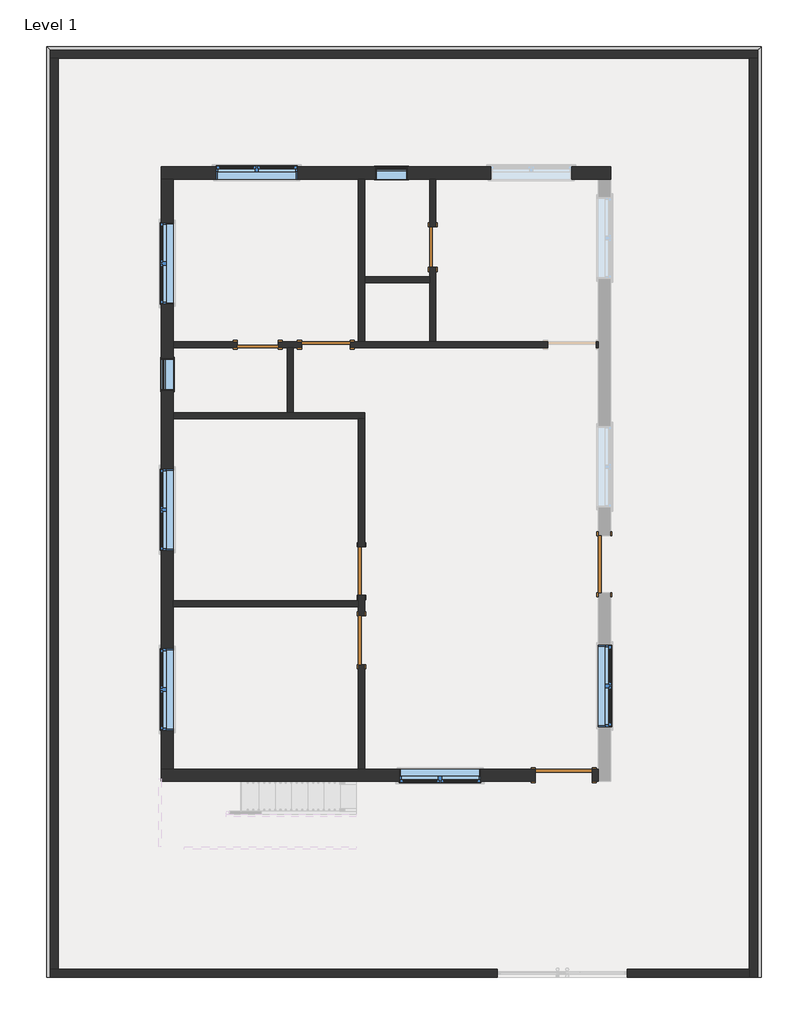
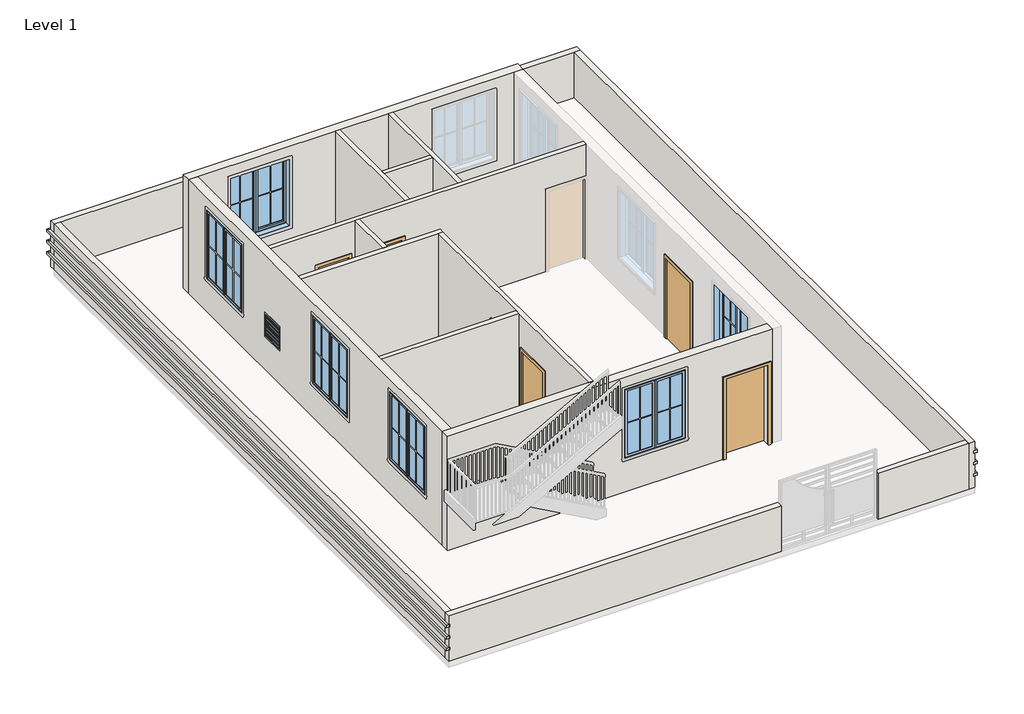
# One storey, part 1 of 3: 16 walls, 8 windows, 7 doors, 3 proxies.
"""IFC4 building model written with IfcOpenShell, lengths in millimetres."""

from ifc_helpers import new_model, si_unit, frame, origin, origin_with_axes, place, context, project, spatial, polyline, outline, extrude, faceted_brep, transform, mapped, element, save
from components import door_78caadf7, single_flush_door_3_e5f9f3c4, single_flush_door_3_305aa2a5, door_9d399b00, door_0848dd25, window_casement_double_win_5_f93960c7, window_f2d8fef0

model = new_model("IFC4")

# Units and contexts
model_context = context("Model", 3, world=origin())
ifc_project = project(units=[si_unit("LENGTHUNIT", "METRE", prefix="MILLI")], contexts=[model_context])

# Site, building, storey
site = spatial("IfcSite", under=ifc_project)
building = spatial("IfcBuilding", under=site)
storey = spatial("IfcBuildingStorey", under=building, Name="Level 1", Elevation=0.0)

# Proxies
placement = place(None, origin())
element("IfcBuildingElementProxy", 1, Name="Reveal", ObjectType="Reveal", at=placement, inside=storey, context=model_context, shape_type="SweptSolid", body=[
    extrude(outline(polyline([(-7520.8438076, -8973.0750537), (-7612.9188076, -8973.0750537), (-7612.9188076, 8467.1999463), (-7520.8438076, 8375.1249463), (-7520.8438076, -8973.0750537)])), frame((0.0, 0.0, 304.8), z_axis=(0.0, 0.0, 1.0), x_axis=(1.0, 0.0, 0.0)), (0.0, 0.0, 1.0), 67.7333333),
    extrude(outline(polyline([(-7520.8438076, 8375.1249463), (-7612.9188076, 8467.1999463), (5779.2311924, 8467.1999463), (5687.1561924, 8375.1249463), (-7520.8438076, 8375.1249463)])), frame((0.0, 0.0, 304.8), z_axis=(0.0, 0.0, 1.0), x_axis=(1.0, 0.0, 0.0)), (0.0, 0.0, 1.0), 67.7333333),
    extrude(outline(polyline([(5687.1561924, 8375.1249463), (5779.2311924, 8467.1999463), (5779.2311924, -8973.0750537), (5687.1561924, -8973.0750537), (5687.1561924, 8375.1249463)])), frame((0.0, 0.0, 304.8), z_axis=(0.0, 0.0, 1.0), x_axis=(1.0, 0.0, 0.0)), (0.0, 0.0, 1.0), 67.7333333),
])
element("IfcBuildingElementProxy", 2, Name="Reveal", ObjectType="Reveal", at=placement, inside=storey, context=model_context, shape_type="SweptSolid", body=[
    extrude(outline(polyline([(-7520.8438076, -8973.0750537), (-7612.9188076, -8973.0750537), (-7612.9188076, 8467.1999463), (-7520.8438076, 8375.1249463), (-7520.8438076, -8973.0750537)])), frame((0.0, 0.0, 609.6), z_axis=(0.0, 0.0, 1.0), x_axis=(1.0, 0.0, 0.0)), (0.0, 0.0, 1.0), 67.7333333),
    extrude(outline(polyline([(-7520.8438076, 8375.1249463), (-7612.9188076, 8467.1999463), (5779.2311924, 8467.1999463), (5687.1561924, 8375.1249463), (-7520.8438076, 8375.1249463)])), frame((0.0, 0.0, 609.6), z_axis=(0.0, 0.0, 1.0), x_axis=(1.0, 0.0, 0.0)), (0.0, 0.0, 1.0), 67.7333333),
    extrude(outline(polyline([(5687.1561924, 8375.1249463), (5779.2311924, 8467.1999463), (5779.2311924, -8973.0750537), (5687.1561924, -8973.0750537), (5687.1561924, 8375.1249463)])), frame((0.0, 0.0, 609.6), z_axis=(0.0, 0.0, 1.0), x_axis=(1.0, 0.0, 0.0)), (0.0, 0.0, 1.0), 67.7333333),
])
element("IfcBuildingElementProxy", 3, Name="Reveal", ObjectType="Reveal", at=placement, inside=storey, context=model_context, shape_type="SweptSolid", body=[
    extrude(outline(polyline([(-7520.8438076, -8973.0750537), (-7612.9188076, -8973.0750537), (-7612.9188076, 8467.1999463), (-7520.8438076, 8375.1249463), (-7520.8438076, -8973.0750537)])), frame((0.0, 0.0, 914.4), z_axis=(0.0, 0.0, 1.0), x_axis=(1.0, 0.0, 0.0)), (0.0, 0.0, 1.0), 67.7333333),
    extrude(outline(polyline([(-7520.8438076, 8375.1249463), (-7612.9188076, 8467.1999463), (5779.2311924, 8467.1999463), (5687.1561924, 8375.1249463), (-7520.8438076, 8375.1249463)])), frame((0.0, 0.0, 914.4), z_axis=(0.0, 0.0, 1.0), x_axis=(1.0, 0.0, 0.0)), (0.0, 0.0, 1.0), 67.7333333),
    extrude(outline(polyline([(5687.1561924, 8375.1249463), (5779.2311924, 8467.1999463), (5779.2311924, -8973.0750537), (5687.1561924, -8973.0750537), (5687.1561924, 8375.1249463)])), frame((0.0, 0.0, 914.4), z_axis=(0.0, 0.0, 1.0), x_axis=(1.0, 0.0, 0.0)), (0.0, 0.0, 1.0), 67.7333333),
])

# Doors
door_shape = door_78caadf7(model_context)
element("IfcDoor", 4, ObjectType="Single-Flush : DOOR 2'6\"", at=placement, inside=storey, context=model_context, shape_type="MappedRepresentation", body=[
    mapped(door_shape, transform((-377.1698569, 4707.5566963, 0.0), x_axis=(0.0, -1.0, 0.0), y_axis=(1.0, 0.0, 0.0), z_axis=(0.0, 0.0, 1.0))),
])
element("IfcDoor", 5, ObjectType="Single-Flush : DOOR 2'6\"", at=placement, inside=storey, context=model_context, shape_type="MappedRepresentation", body=[
    mapped(door_shape, transform((-3653.7698569, 2878.7566963, 0.0), x_axis=(1.0, 0.0, 0.0), y_axis=(0.0, 1.0, 0.0), z_axis=(0.0, 0.0, 1.0))),
])
single_flush_door_3_shape = single_flush_door_3_e5f9f3c4(model_context)
element("IfcDoor", 6, ObjectType="Single-Flush : DOOR 3'", at=placement, inside=storey, context=model_context, shape_type="MappedRepresentation", body=[
    mapped(single_flush_door_3_shape, transform((-2377.4198569, 2878.7566963, 0.0), x_axis=(1.0, 0.0, 0.0), y_axis=(0.0, 1.0, 0.0), z_axis=(0.0, 0.0, 1.0))),
])
element("IfcDoor", 7, ObjectType="Single-Flush : DOOR 3'", at=placement, inside=storey, context=model_context, shape_type="MappedRepresentation", body=[
    mapped(single_flush_door_3_shape, transform((-1710.6698569, -2658.4433037, 0.0), x_axis=(0.0, 1.0, 0.0), y_axis=(-1.0, 0.0, 0.0), z_axis=(0.0, 0.0, 1.0))),
])
single_flush_door_3_2_shape = single_flush_door_3_305aa2a5(model_context)
element("IfcDoor", 8, ObjectType="Single-Flush : DOOR 3'", at=placement, inside=storey, context=model_context, shape_type="MappedRepresentation", body=[
    mapped(single_flush_door_3_2_shape, transform((-1710.6698569, -1363.0433037, 0.0), x_axis=(0.0, -1.0, 0.0), y_axis=(1.0, 0.0, 0.0), z_axis=(0.0, 0.0, 1.0))),
])
door_2_shape = door_9d399b00(model_context)
element("IfcDoor", 9, ObjectType="Single-Flush : DOOR 3'6\"", at=placement, inside=storey, context=model_context, shape_type="MappedRepresentation", body=[
    mapped(door_2_shape, transform((2080.2801431, -5192.0933037, 0.0), x_axis=(1.0, 0.0, 0.0), y_axis=(0.0, 1.0, 0.0), z_axis=(0.0, 0.0, 1.0))),
])
door_3_shape = door_0848dd25(model_context)
element("IfcDoor", 10, ObjectType="Single-Flush : DOOR 3'6\"", at=placement, inside=storey, context=model_context, shape_type="MappedRepresentation", body=[
    mapped(door_3_shape, transform((2842.2801431, -1236.0433037, 0.0), x_axis=(0.0, -1.0, 0.0), y_axis=(1.0, 0.0, 0.0), z_axis=(0.0, 0.0, 1.0))),
])

# Walls
element("IfcWall", 11, ObjectType="CMD 6\"", at=placement, inside=storey, context=model_context, shape_type="Brep", body=[
    faceted_brep([(-7546.2438076, 8248.1249463, 0.0), (-7393.8438076, 8248.1249463, 0.0), (5560.1561924, 8248.1249463, 0.0), (5712.5561924, 8248.1249463, 0.0), (5712.5561924, 8248.1249463, 304.8), (5687.1561924, 8248.1249463, 304.8), (5687.1561924, 8248.1249463, 372.5333333), (5712.5561924, 8248.1249463, 372.5333333), (5712.5561924, 8248.1249463, 609.6), (5687.1561924, 8248.1249463, 609.6), (5687.1561924, 8248.1249463, 677.3333333), (5712.5561924, 8248.1249463, 677.3333333), (5712.5561924, 8248.1249463, 914.4), (5687.1561924, 8248.1249463, 914.4), (5687.1561924, 8248.1249463, 982.1333333), (5712.5561924, 8248.1249463, 982.1333333), (5712.5561924, 8248.1249463, 1219.2), (5560.1561924, 8248.1249463, 1219.2), (-7393.8438076, 8248.1249463, 1219.2), (-7546.2438076, 8248.1249463, 1219.2), (-7546.2438076, 8248.1249463, 982.1333333), (-7520.8438076, 8248.1249463, 982.1333333), (-7520.8438076, 8248.1249463, 914.4), (-7546.2438076, 8248.1249463, 914.4), (-7546.2438076, 8248.1249463, 677.3333333), (-7520.8438076, 8248.1249463, 677.3333333), (-7520.8438076, 8248.1249463, 609.6), (-7546.2438076, 8248.1249463, 609.6), (-7546.2438076, 8248.1249463, 372.5333333), (-7520.8438076, 8248.1249463, 372.5333333), (-7520.8438076, 8248.1249463, 304.8), (-7546.2438076, 8248.1249463, 304.8), (5712.5561924, 8400.5249463, 0.0), (-7546.2438076, 8400.5249463, 0.0), (-7546.2438076, 8400.5249463, 304.8), (5712.5561924, 8400.5249463, 304.8), (-7546.2438076, 8400.5249463, 1219.2), (5712.5561924, 8400.5249463, 1219.2), (5712.5561924, 8400.5249463, 982.1333333), (-7546.2438076, 8400.5249463, 982.1333333), (5712.5561924, 8400.5249463, 372.5333333), (-7546.2438076, 8400.5249463, 372.5333333), (-7546.2438076, 8400.5249463, 609.6), (5712.5561924, 8400.5249463, 609.6), (5712.5561924, 8400.5249463, 677.3333333), (-7546.2438076, 8400.5249463, 677.3333333), (-7546.2438076, 8400.5249463, 914.4), (5712.5561924, 8400.5249463, 914.4), (5687.1561924, 8375.1249463, 372.5333333), (-7520.8438076, 8375.1249463, 372.5333333), (-7520.8438076, 8375.1249463, 304.8), (5687.1561924, 8375.1249463, 304.8), (5687.1561924, 8375.1249463, 677.3333333), (-7520.8438076, 8375.1249463, 677.3333333), (-7520.8438076, 8375.1249463, 609.6), (5687.1561924, 8375.1249463, 609.6), (5687.1561924, 8375.1249463, 982.1333333), (-7520.8438076, 8375.1249463, 982.1333333), (-7520.8438076, 8375.1249463, 914.4), (5687.1561924, 8375.1249463, 914.4)], [[[0, 1, 2, 3, 4, 5, 6, 7, 8, 9, 10, 11, 12, 13, 14, 15, 16, 17, 18, 19, 20, 21, 22, 23, 24, 25, 26, 27, 28, 29, 30, 31]], [[32, 33, 34, 35]], [[36, 37, 38, 39]], [[40, 41, 42, 43]], [[44, 45, 46, 47]], [[3, 2, 1, 0, 33, 32]], [[19, 18, 17, 16, 37, 36]], [[3, 32, 35, 4]], [[37, 16, 15, 38]], [[7, 40, 43, 8]], [[11, 44, 47, 12]], [[19, 36, 39, 20]], [[33, 0, 31, 34]], [[41, 28, 27, 42]], [[45, 24, 23, 46]], [[48, 49, 29, 28, 41, 40, 7, 6]], [[50, 51, 5, 4, 35, 34, 31, 30]], [[49, 50, 30, 29]], [[49, 48, 51, 50]], [[51, 48, 6, 5]], [[52, 53, 25, 24, 45, 44, 11, 10]], [[54, 55, 9, 8, 43, 42, 27, 26]], [[53, 54, 26, 25]], [[53, 52, 55, 54]], [[55, 52, 10, 9]], [[56, 57, 21, 20, 39, 38, 15, 14]], [[58, 59, 13, 12, 47, 46, 23, 22]], [[57, 58, 22, 21]], [[57, 56, 59, 58]], [[59, 56, 14, 13]]]),
])
element("IfcWall", 12, ObjectType="CMD 6\"", at=placement, inside=storey, context=model_context, shape_type="Brep", body=[
    faceted_brep([(5560.1561924, 8248.1249463, 0.0), (5560.1561924, -8820.6750537, 0.0), (5560.1561924, -8973.0750537, 0.0), (5560.1561924, -8973.0750537, 1219.2), (5560.1561924, -8820.6750537, 1219.2), (5560.1561924, 8248.1249463, 1219.2), (5712.5561924, -8973.0750537, 0.0), (5712.5561924, 8248.1249463, 0.0), (5712.5561924, 8248.1249463, 304.8), (5712.5561924, -8973.0750537, 304.8), (5712.5561924, 8248.1249463, 1219.2), (5712.5561924, -8973.0750537, 1219.2), (5712.5561924, -8973.0750537, 982.1333333), (5712.5561924, 8248.1249463, 982.1333333), (5712.5561924, -8973.0750537, 372.5333333), (5712.5561924, 8248.1249463, 372.5333333), (5712.5561924, 8248.1249463, 609.6), (5712.5561924, -8973.0750537, 609.6), (5712.5561924, -8973.0750537, 677.3333333), (5712.5561924, 8248.1249463, 677.3333333), (5712.5561924, 8248.1249463, 914.4), (5712.5561924, -8973.0750537, 914.4), (5687.1561924, 8248.1249463, 982.1333333), (5687.1561924, 8248.1249463, 914.4), (5687.1561924, 8248.1249463, 677.3333333), (5687.1561924, 8248.1249463, 609.6), (5687.1561924, 8248.1249463, 372.5333333), (5687.1561924, 8248.1249463, 304.8), (5687.1561924, -8973.0750537, 304.8), (5687.1561924, -8973.0750537, 372.5333333), (5687.1561924, -8973.0750537, 609.6), (5687.1561924, -8973.0750537, 677.3333333), (5687.1561924, -8973.0750537, 914.4), (5687.1561924, -8973.0750537, 982.1333333)], [[[0, 1, 2, 3, 4, 5]], [[6, 7, 8, 9]], [[10, 11, 12, 13]], [[14, 15, 16, 17]], [[18, 19, 20, 21]], [[2, 1, 0, 7, 6]], [[5, 4, 3, 11, 10]], [[0, 5, 10, 13, 22, 23, 20, 19, 24, 25, 16, 15, 26, 27, 8, 7]], [[3, 2, 6, 9, 28, 29, 14, 17, 30, 31, 18, 21, 32, 33, 12, 11]], [[29, 26, 15, 14]], [[27, 28, 9, 8]], [[26, 29, 28, 27]], [[31, 24, 19, 18]], [[25, 30, 17, 16]], [[24, 31, 30, 25]], [[33, 22, 13, 12]], [[23, 32, 21, 20]], [[22, 33, 32, 23]]]),
])
element("IfcWall", 13, ObjectType="CMD 6\"", at=placement, inside=storey, context=model_context, shape_type="SweptSolid", body=[
    extrude(outline(polyline([(3274.1561924, -8820.6750537), (5560.1561924, -8820.6750537), (5560.1561924, -8973.0750537), (3274.1561924, -8973.0750537), (3274.1561924, -8820.6750537)])), origin_with_axes(), (0.0, 0.0, 1.0), 1219.2),
])
element("IfcWall", 14, ObjectType="CMD 6\"", at=placement, inside=storey, context=model_context, shape_type="SweptSolid", body=[
    extrude(outline(polyline([(0.0, -7393.8438076), (1219.2, -7393.8438076), (1219.2, -7546.2438076), (982.1333333, -7546.2438076), (982.1333333, -7520.8438076), (914.4, -7520.8438076), (914.4, -7546.2438076), (677.3333333, -7546.2438076), (677.3333333, -7520.8438076), (609.6, -7520.8438076), (609.6, -7546.2438076), (372.5333333, -7546.2438076), (372.5333333, -7520.8438076), (304.8, -7520.8438076), (304.8, -7546.2438076), (0.0, -7546.2438076), (0.0, -7393.8438076)])), frame((0.0, -8820.6750537, 0.0), z_axis=(0.0, 1.0, 0.0), x_axis=(0.0, 0.0, 1.0)), (0.0, 0.0, 1.0), 17068.8),
])
element("IfcWall", 15, ObjectType="CMD 6\"", at=placement, inside=storey, context=model_context, shape_type="Brep", body=[
    faceted_brep([(835.7561924, -8820.6750537, 0.0), (-7393.8438076, -8820.6750537, 0.0), (-7546.2438076, -8820.6750537, 0.0), (-7546.2438076, -8820.6750537, 304.8), (-7520.8438076, -8820.6750537, 304.8), (-7520.8438076, -8820.6750537, 372.5333333), (-7546.2438076, -8820.6750537, 372.5333333), (-7546.2438076, -8820.6750537, 609.6), (-7520.8438076, -8820.6750537, 609.6), (-7520.8438076, -8820.6750537, 677.3333333), (-7546.2438076, -8820.6750537, 677.3333333), (-7546.2438076, -8820.6750537, 914.4), (-7520.8438076, -8820.6750537, 914.4), (-7520.8438076, -8820.6750537, 982.1333333), (-7546.2438076, -8820.6750537, 982.1333333), (-7546.2438076, -8820.6750537, 1219.2), (-7393.8438076, -8820.6750537, 1219.2), (835.7561924, -8820.6750537, 1219.2), (-7546.2438076, -8973.0750537, 0.0), (835.7561924, -8973.0750537, 0.0), (835.7561924, -8973.0750537, 1219.2), (-7546.2438076, -8973.0750537, 1219.2), (-7546.2438076, -8973.0750537, 982.1333333), (-7520.8438076, -8973.0750537, 982.1333333), (-7520.8438076, -8973.0750537, 914.4), (-7546.2438076, -8973.0750537, 914.4), (-7546.2438076, -8973.0750537, 677.3333333), (-7520.8438076, -8973.0750537, 677.3333333), (-7520.8438076, -8973.0750537, 609.6), (-7546.2438076, -8973.0750537, 609.6), (-7546.2438076, -8973.0750537, 372.5333333), (-7520.8438076, -8973.0750537, 372.5333333), (-7520.8438076, -8973.0750537, 304.8), (-7546.2438076, -8973.0750537, 304.8)], [[[0, 1, 2, 3, 4, 5, 6, 7, 8, 9, 10, 11, 12, 13, 14, 15, 16, 17]], [[18, 19, 20, 21, 22, 23, 24, 25, 26, 27, 28, 29, 30, 31, 32, 33]], [[2, 1, 0, 19, 18]], [[17, 16, 15, 21, 20]], [[0, 17, 20, 19]], [[2, 18, 33, 3]], [[21, 15, 14, 22]], [[6, 30, 29, 7]], [[10, 26, 25, 11]], [[5, 31, 30, 6]], [[32, 4, 3, 33]], [[31, 5, 4, 32]], [[9, 27, 26, 10]], [[28, 8, 7, 29]], [[27, 9, 8, 28]], [[13, 23, 22, 14]], [[24, 12, 11, 25]], [[23, 13, 12, 24]]]),
])
element("IfcWall", 16, ObjectType="WALL 4.5\"", at=placement, inside=storey, context=model_context, shape_type="Brep", body=[
    faceted_brep([(2689.8801431, 2821.6066963, 2133.6), (2689.8801431, 2821.6066963, 0.0), (2727.9801431, 2821.6066963, 0.0), (2727.9801431, 2821.6066963, 3048.0), (-2987.0198569, 2821.6066963, 3048.0), (-3101.3198569, 2821.6066963, 3048.0), (-5234.9198569, 2821.6066963, 3048.0), (-5234.9198569, 2821.6066963, 0.0), (-4034.7698569, 2821.6066963, 0.0), (-4034.7698569, 2821.6066963, 2133.6), (-3272.7698569, 2821.6066963, 2133.6), (-3272.7698569, 2821.6066963, 0.0), (-3101.3198569, 2821.6066963, 0.0), (-2987.0198569, 2821.6066963, 0.0), (-2834.6198569, 2821.6066963, 0.0), (-2834.6198569, 2821.6066963, 2133.6), (-1920.2198569, 2821.6066963, 2133.6), (-1920.2198569, 2821.6066963, 0.0), (1775.4801431, 2821.6066963, 0.0), (1775.4801431, 2821.6066963, 2133.6), (2727.9801431, 2935.9066963, 0.0), (2689.8801431, 2935.9066963, 0.0), (2689.8801431, 2935.9066963, 2133.6), (1775.4801431, 2935.9066963, 2133.6), (1775.4801431, 2935.9066963, 0.0), (-320.0198569, 2935.9066963, 0.0), (-434.3198569, 2935.9066963, 0.0), (-1653.5198569, 2935.9066963, 0.0), (-1767.8198569, 2935.9066963, 0.0), (-1920.2198569, 2935.9066963, 0.0), (-1920.2198569, 2935.9066963, 2133.6), (-2834.6198569, 2935.9066963, 2133.6), (-2834.6198569, 2935.9066963, 0.0), (-3272.7698569, 2935.9066963, 0.0), (-3272.7698569, 2935.9066963, 2133.6), (-4034.7698569, 2935.9066963, 2133.6), (-4034.7698569, 2935.9066963, 0.0), (-5234.9198569, 2935.9066963, 0.0), (-5234.9198569, 2935.9066963, 3048.0), (-1767.8198569, 2935.9066963, 3048.0), (-1653.5198569, 2935.9066963, 3048.0), (-434.3198569, 2935.9066963, 3048.0), (-320.0198569, 2935.9066963, 3048.0), (2727.9801431, 2935.9066963, 3048.0)], [[[0, 1, 2, 3, 4, 5, 6, 7, 8, 9, 10, 11, 12, 13, 14, 15, 16, 17, 18, 19]], [[20, 21, 22, 23, 24, 25, 26, 27, 28, 29, 30, 31, 32, 33, 34, 35, 36, 37, 38, 39, 40, 41, 42, 43]], [[8, 7, 37, 36]], [[14, 13, 12, 11, 33, 32]], [[18, 17, 29, 28, 27, 26, 25, 24]], [[2, 1, 21, 20]], [[3, 2, 20, 43]], [[7, 6, 38, 37]], [[34, 33, 11, 10]], [[35, 34, 10, 9]], [[36, 35, 9, 8]], [[30, 29, 17, 16]], [[31, 30, 16, 15]], [[32, 31, 15, 14]], [[22, 21, 1, 0]], [[23, 22, 0, 19]], [[24, 23, 19, 18]], [[6, 5, 4, 3, 43, 42, 41, 40, 39, 38]]]),
])
element("IfcWall", 17, ObjectType="WALL 4.5\"", at=placement, inside=storey, context=model_context, shape_type="Brep", body=[
    faceted_brep([(-1767.8198569, 5983.9066963, 0.0), (-1767.8198569, 2935.9066963, 0.0), (-1767.8198569, 2935.9066963, 3048.0), (-1767.8198569, 5983.9066963, 3048.0), (-1653.5198569, 5983.9066963, 0.0), (-1653.5198569, 5983.9066963, 3048.0), (-1653.5198569, 4155.1066963, 3048.0), (-1653.5198569, 4040.8066963, 3048.0), (-1653.5198569, 2935.9066963, 3048.0), (-1653.5198569, 2935.9066963, 0.0), (-1653.5198569, 4040.8066963, 0.0), (-1653.5198569, 4155.1066963, 0.0)], [[[0, 1, 2, 3]], [[4, 5, 6, 7, 8, 9, 10, 11]], [[1, 0, 4, 11, 10, 9]], [[0, 3, 5, 4]], [[2, 1, 9, 8]], [[3, 2, 8, 7, 6, 5]]]),
])
element("IfcWall", 18, ObjectType="WALL 4.5\"", at=placement, inside=storey, context=model_context, shape_type="Brep", body=[
    faceted_brep([(-320.0198569, 2935.9066963, 0.0), (-320.0198569, 4326.5566963, 0.0), (-320.0198569, 4326.5566963, 2133.6), (-320.0198569, 5088.5566963, 2133.6), (-320.0198569, 5088.5566963, 0.0), (-320.0198569, 5983.9066963, 0.0), (-320.0198569, 5983.9066963, 3048.0), (-320.0198569, 2935.9066963, 3048.0), (-434.3198569, 4326.5566963, 2133.6), (-434.3198569, 4326.5566963, 0.0), (-434.3198569, 4155.1066963, 0.0), (-434.3198569, 4040.8066963, 0.0), (-434.3198569, 2935.9066963, 0.0), (-434.3198569, 2935.9066963, 3048.0), (-434.3198569, 4040.8066963, 3048.0), (-434.3198569, 4155.1066963, 3048.0), (-434.3198569, 5983.9066963, 3048.0), (-434.3198569, 5983.9066963, 0.0), (-434.3198569, 5088.5566963, 0.0), (-434.3198569, 5088.5566963, 2133.6)], [[[0, 1, 2, 3, 4, 5, 6, 7]], [[8, 9, 10, 11, 12, 13, 14, 15, 16, 17, 18, 19]], [[18, 17, 5, 4]], [[12, 11, 10, 9, 1, 0]], [[6, 5, 17, 16]], [[0, 7, 13, 12]], [[2, 1, 9, 8]], [[3, 2, 8, 19]], [[4, 3, 19, 18]], [[7, 6, 16, 15, 14, 13]]]),
])
element("IfcWall", 19, ObjectType="WALL 4.5\"", at=placement, inside=storey, context=model_context, shape_type="SweptSolid", body=[
    extrude(outline(polyline([(-434.3198569, 4040.8066963), (-1653.5198569, 4040.8066963), (-1653.5198569, 4155.1066963), (-434.3198569, 4155.1066963), (-434.3198569, 4040.8066963)])), origin_with_axes(), (0.0, 0.0, 1.0), 3048.0),
])
element("IfcWall", 20, ObjectType="WALL 4.5\"", at=placement, inside=storey, context=model_context, shape_type="Brep", body=[
    faceted_brep([(-5234.9198569, 1488.1066963, 0.0), (-1767.8198569, 1488.1066963, 0.0), (-1653.5198569, 1488.1066963, 0.0), (-1653.5198569, 1488.1066963, 3048.0), (-1767.8198569, 1488.1066963, 3048.0), (-5234.9198569, 1488.1066963, 3048.0), (-5234.9198569, 1602.4066963, 0.0), (-5234.9198569, 1602.4066963, 3048.0), (-3101.3198569, 1602.4066963, 3048.0), (-2987.0198569, 1602.4066963, 3048.0), (-1653.5198569, 1602.4066963, 3048.0), (-1653.5198569, 1602.4066963, 0.0), (-2987.0198569, 1602.4066963, 0.0), (-3101.3198569, 1602.4066963, 0.0)], [[[0, 1, 2, 3, 4, 5]], [[6, 7, 8, 9, 10, 11, 12, 13]], [[2, 1, 0, 6, 13, 12, 11]], [[0, 5, 7, 6]], [[3, 2, 11, 10]], [[5, 4, 3, 10, 9, 8, 7]]]),
])
element("IfcWall", 21, ObjectType="WALL 4.5\"", at=placement, inside=storey, context=model_context, shape_type="Brep", body=[
    faceted_brep([(-1767.8198569, -1820.2433037, 0.0), (-1767.8198569, -1915.4933037, 0.0), (-1767.8198569, -2029.7933037, 0.0), (-1767.8198569, -2201.2433037, 0.0), (-1767.8198569, -2201.2433037, 2133.6), (-1767.8198569, -3115.6433037, 2133.6), (-1767.8198569, -3115.6433037, 0.0), (-1767.8198569, -5077.7933037, 0.0), (-1767.8198569, -5077.7933037, 3048.0), (-1767.8198569, -2029.7933037, 3048.0), (-1767.8198569, -1915.4933037, 3048.0), (-1767.8198569, 1488.1066963, 3048.0), (-1767.8198569, 1488.1066963, 0.0), (-1767.8198569, -905.8433037, 0.0), (-1767.8198569, -905.8433037, 2133.6), (-1767.8198569, -1820.2433037, 2133.6), (-1653.5198569, -2201.2433037, 2133.6), (-1653.5198569, -2201.2433037, 0.0), (-1653.5198569, -1820.2433037, 0.0), (-1653.5198569, -1820.2433037, 2133.6), (-1653.5198569, -905.8433037, 2133.6), (-1653.5198569, -905.8433037, 0.0), (-1653.5198569, 1488.1066963, 0.0), (-1653.5198569, 1488.1066963, 3048.0), (-1653.5198569, -5077.7933037, 3048.0), (-1653.5198569, -5077.7933037, 0.0), (-1653.5198569, -3115.6433037, 0.0), (-1653.5198569, -3115.6433037, 2133.6)], [[[0, 1, 2, 3, 4, 5, 6, 7, 8, 9, 10, 11, 12, 13, 14, 15]], [[16, 17, 18, 19, 20, 21, 22, 23, 24, 25, 26, 27]], [[13, 12, 22, 21]], [[26, 25, 7, 6]], [[18, 17, 3, 2, 1, 0]], [[12, 11, 23, 22]], [[8, 7, 25, 24]], [[19, 18, 0, 15]], [[20, 19, 15, 14]], [[21, 20, 14, 13]], [[4, 3, 17, 16]], [[5, 4, 16, 27]], [[6, 5, 27, 26]], [[11, 10, 9, 8, 24, 23]]]),
])
element("IfcWall", 22, ObjectType="WALL 4.5\"", at=placement, inside=storey, context=model_context, shape_type="SweptSolid", body=[
    extrude(outline(polyline([(-1767.8198569, -2029.7933037), (-5234.9198569, -2029.7933037), (-5234.9198569, -1915.4933037), (-1767.8198569, -1915.4933037), (-1767.8198569, -2029.7933037)])), origin_with_axes(), (0.0, 0.0, 1.0), 3048.0),
])
element("IfcWall", 23, ObjectType="WALL 4.5\"", at=placement, inside=storey, context=model_context, shape_type="SweptSolid", body=[
    extrude(outline(polyline([(-3101.3198569, 1602.4066963), (-3101.3198569, 2821.6066963), (-2987.0198569, 2821.6066963), (-2987.0198569, 1602.4066963), (-3101.3198569, 1602.4066963)])), origin_with_axes(), (0.0, 0.0, 1.0), 3048.0),
])
element("IfcWall", 24, ObjectType="WALL 9\"", at=placement, inside=storey, context=model_context, shape_type="Brep", body=[
    faceted_brep([(-5463.5198569, 5983.9066963, 0.0), (-5234.9198569, 5983.9066963, 0.0), (-1767.8198569, 5983.9066963, 0.0), (-1653.5198569, 5983.9066963, 0.0), (-434.3198569, 5983.9066963, 0.0), (-320.0198569, 5983.9066963, 0.0), (2727.9801431, 5983.9066963, 0.0), (2956.5801431, 5983.9066963, 0.0), (2956.5801431, 5983.9066963, 3048.0), (2727.9801431, 5983.9066963, 3048.0), (-320.0198569, 5983.9066963, 3048.0), (-434.3198569, 5983.9066963, 3048.0), (-1653.5198569, 5983.9066963, 3048.0), (-1767.8198569, 5983.9066963, 3048.0), (-5234.9198569, 5983.9066963, 3048.0), (-5463.5198569, 5983.9066963, 3048.0), (2232.6801431, 5983.9066963, 2743.2), (2232.6801431, 5983.9066963, 914.4), (708.6801431, 5983.9066963, 914.4), (708.6801431, 5983.9066963, 2743.2), (-2910.8198569, 5983.9066963, 2743.2), (-2910.8198569, 5983.9066963, 914.4), (-4434.8198569, 5983.9066963, 914.4), (-4434.8198569, 5983.9066963, 2743.2), (-1456.6698569, 5983.9066963, 1524.0), (-847.0698569, 5983.9066963, 1524.0), (-847.0698569, 5983.9066963, 914.4), (-1456.6698569, 5983.9066963, 914.4), (-5463.5198569, 6212.5066963, 0.0), (-5463.5198569, 6212.5066963, 3048.0), (2956.5801431, 6212.5066963, 3048.0), (2956.5801431, 6212.5066963, 0.0), (2232.6801431, 6212.5066963, 2743.2), (708.6801431, 6212.5066963, 2743.2), (708.6801431, 6212.5066963, 914.4), (2232.6801431, 6212.5066963, 914.4), (-2910.8198569, 6212.5066963, 2743.2), (-4434.8198569, 6212.5066963, 2743.2), (-4434.8198569, 6212.5066963, 914.4), (-2910.8198569, 6212.5066963, 914.4), (-1456.6698569, 6212.5066963, 1524.0), (-1456.6698569, 6212.5066963, 914.4), (-847.0698569, 6212.5066963, 914.4), (-847.0698569, 6212.5066963, 1524.0)], [[[0, 1, 2, 3, 4, 5, 6, 7, 8, 9, 10, 11, 12, 13, 14, 15], [16, 17, 18, 19], [20, 21, 22, 23], [24, 25, 26, 27]], [[28, 29, 30, 31], [32, 33, 34, 35], [36, 37, 38, 39], [40, 41, 42, 43]], [[7, 6, 5, 4, 3, 2, 1, 0, 28, 31]], [[8, 7, 31, 30]], [[0, 15, 29, 28]], [[17, 16, 32, 35]], [[18, 17, 35, 34]], [[19, 18, 34, 33]], [[16, 19, 33, 32]], [[21, 20, 36, 39]], [[22, 21, 39, 38]], [[23, 22, 38, 37]], [[20, 23, 37, 36]], [[41, 40, 24, 27]], [[42, 41, 27, 26]], [[43, 42, 26, 25]], [[40, 43, 25, 24]], [[15, 14, 13, 12, 11, 10, 9, 8, 30, 29]]]),
])
element("IfcWall", 25, ObjectType="WALL 9\"", at=placement, inside=storey, context=model_context, shape_type="Brep", body=[
    faceted_brep([(2727.9801431, -5077.7933037, 0.0), (2613.6801431, -5077.7933037, 0.0), (2613.6801431, -5077.7933037, 2133.6), (1546.8801431, -5077.7933037, 2133.6), (1546.8801431, -5077.7933037, 0.0), (-1653.5198569, -5077.7933037, 0.0), (-1767.8198569, -5077.7933037, 0.0), (-5234.9198569, -5077.7933037, 0.0), (-5463.5198569, -5077.7933037, 0.0), (-5463.5198569, -5077.7933037, 3048.0), (-5234.9198569, -5077.7933037, 3048.0), (-1767.8198569, -5077.7933037, 3048.0), (-1653.5198569, -5077.7933037, 3048.0), (2727.9801431, -5077.7933037, 3048.0), (-999.4698569, -5077.7933037, 2743.2), (-999.4698569, -5077.7933037, 914.4), (524.5301431, -5077.7933037, 914.4), (524.5301431, -5077.7933037, 2743.2), (2613.6801431, -5306.3933037, 2133.6), (2613.6801431, -5306.3933037, 0.0), (2727.9801431, -5306.3933037, 0.0), (2727.9801431, -5306.3933037, 3048.0), (-1831.3198569, -5306.3933037, 3048.0), (-5463.5198569, -5306.3933037, 3048.0), (-5463.5198569, -5306.3933037, 0.0), (1546.8801431, -5306.3933037, 0.0), (1546.8801431, -5306.3933037, 2133.6), (-999.4698569, -5306.3933037, 2743.2), (524.5301431, -5306.3933037, 2743.2), (524.5301431, -5306.3933037, 914.4), (-999.4698569, -5306.3933037, 914.4)], [[[0, 1, 2, 3, 4, 5, 6, 7, 8, 9, 10, 11, 12, 13], [14, 15, 16, 17]], [[18, 19, 20, 21, 22, 23, 24, 25, 26], [27, 28, 29, 30]], [[25, 24, 8, 7, 6, 5, 4]], [[20, 19, 1, 0]], [[0, 13, 21, 20]], [[9, 8, 24, 23]], [[15, 14, 27, 30]], [[16, 15, 30, 29]], [[17, 16, 29, 28]], [[14, 17, 28, 27]], [[2, 1, 19, 18]], [[3, 2, 18, 26]], [[4, 3, 26, 25]], [[13, 12, 11, 10, 9, 23, 22, 21]]]),
])
element("IfcWall", 26, ObjectType="WALL 9\"", at=placement, inside=storey, context=model_context, shape_type="Brep", body=[
    faceted_brep([(-5234.9198569, -5077.7933037, 0.0), (-5234.9198569, -2029.7933037, 0.0), (-5234.9198569, -1915.4933037, 0.0), (-5234.9198569, 1488.1066963, 0.0), (-5234.9198569, 1602.4066963, 0.0), (-5234.9198569, 2821.6066963, 0.0), (-5234.9198569, 2935.9066963, 0.0), (-5234.9198569, 5983.9066963, 0.0), (-5234.9198569, 5983.9066963, 3048.0), (-5234.9198569, 2935.9066963, 3048.0), (-5234.9198569, 2821.6066963, 3048.0), (-5234.9198569, 1602.4066963, 3048.0), (-5234.9198569, 1488.1066963, 3048.0), (-5234.9198569, -1915.4933037, 3048.0), (-5234.9198569, -2029.7933037, 3048.0), (-5234.9198569, -5077.7933037, 3048.0), (-5234.9198569, -2820.3683037, 2743.2), (-5234.9198569, -2820.3683037, 914.4), (-5234.9198569, -4344.3683037, 914.4), (-5234.9198569, -4344.3683037, 2743.2), (-5234.9198569, 548.3066963, 2743.2), (-5234.9198569, 548.3066963, 914.4), (-5234.9198569, -975.6933037, 914.4), (-5234.9198569, -975.6933037, 2743.2), (-5234.9198569, 5164.7566963, 2743.2), (-5234.9198569, 5164.7566963, 914.4), (-5234.9198569, 3640.7566963, 914.4), (-5234.9198569, 3640.7566963, 2743.2), (-5234.9198569, 2015.1566963, 1524.0), (-5234.9198569, 2624.7566963, 1524.0), (-5234.9198569, 2624.7566963, 914.4), (-5234.9198569, 2015.1566963, 914.4), (-5463.5198569, -5077.7933037, 0.0), (-5463.5198569, -5077.7933037, 3048.0), (-5463.5198569, 5983.9066963, 3048.0), (-5463.5198569, 5983.9066963, 0.0), (-5463.5198569, -2820.3683037, 2743.2), (-5463.5198569, -4344.3683037, 2743.2), (-5463.5198569, -4344.3683037, 914.4), (-5463.5198569, -2820.3683037, 914.4), (-5463.5198569, 548.3066963, 2743.2), (-5463.5198569, -975.6933037, 2743.2), (-5463.5198569, -975.6933037, 914.4), (-5463.5198569, 548.3066963, 914.4), (-5463.5198569, 5164.7566963, 2743.2), (-5463.5198569, 3640.7566963, 2743.2), (-5463.5198569, 3640.7566963, 914.4), (-5463.5198569, 5164.7566963, 914.4), (-5463.5198569, 2015.1566963, 1524.0), (-5463.5198569, 2015.1566963, 914.4), (-5463.5198569, 2624.7566963, 914.4), (-5463.5198569, 2624.7566963, 1524.0)], [[[0, 1, 2, 3, 4, 5, 6, 7, 8, 9, 10, 11, 12, 13, 14, 15], [16, 17, 18, 19], [20, 21, 22, 23], [24, 25, 26, 27], [28, 29, 30, 31]], [[32, 33, 34, 35], [36, 37, 38, 39], [40, 41, 42, 43], [44, 45, 46, 47], [48, 49, 50, 51]], [[7, 6, 5, 4, 3, 2, 1, 0, 32, 35]], [[8, 7, 35, 34]], [[0, 15, 33, 32]], [[17, 16, 36, 39]], [[18, 17, 39, 38]], [[19, 18, 38, 37]], [[16, 19, 37, 36]], [[21, 20, 40, 43]], [[22, 21, 43, 42]], [[23, 22, 42, 41]], [[20, 23, 41, 40]], [[25, 24, 44, 47]], [[26, 25, 47, 46]], [[27, 26, 46, 45]], [[24, 27, 45, 44]], [[49, 48, 28, 31]], [[50, 49, 31, 30]], [[51, 50, 30, 29]], [[48, 51, 29, 28]], [[15, 14, 13, 12, 11, 10, 9, 8, 34, 33]]]),
])

# Windows
window_casement_double_win_5_shape = window_casement_double_win_5_f93960c7(model_context)
element("IfcWindow", 27, ObjectType="Window-Casement-Double : WIN 5'", at=placement, inside=storey, context=model_context, shape_type="MappedRepresentation", body=[
    mapped(window_casement_double_win_5_shape, transform((-5349.2198569, -3582.3683037, 0.0), x_axis=(0.0, 1.0, 0.0), y_axis=(-1.0, 0.0, 0.0), z_axis=(0.0, 0.0, 1.0))),
])
element("IfcWindow", 28, ObjectType="Window-Casement-Double : WIN 5'", at=placement, inside=storey, context=model_context, shape_type="MappedRepresentation", body=[
    mapped(window_casement_double_win_5_shape, transform((-5349.2198569, -213.6933037, 0.0), x_axis=(0.0, 1.0, 0.0), y_axis=(-1.0, 0.0, 0.0), z_axis=(0.0, 0.0, 1.0))),
])
element("IfcWindow", 29, ObjectType="Window-Casement-Double : WIN 5'", at=placement, inside=storey, context=model_context, shape_type="MappedRepresentation", body=[
    mapped(window_casement_double_win_5_shape, transform((-5349.2198569, 4402.7566963, 0.0), x_axis=(0.0, 1.0, 0.0), y_axis=(-1.0, 0.0, 0.0), z_axis=(0.0, 0.0, 1.0))),
])
element("IfcWindow", 30, ObjectType="Window-Casement-Double : WIN 5'", at=placement, inside=storey, context=model_context, shape_type="MappedRepresentation", body=[
    mapped(window_casement_double_win_5_shape, transform((2842.2801431, -3515.6933037, 0.0), x_axis=(0.0, -1.0, 0.0), y_axis=(1.0, 0.0, 0.0), z_axis=(0.0, 0.0, 1.0))),
])
element("IfcWindow", 31, ObjectType="Window-Casement-Double : WIN 5'", at=placement, inside=storey, context=model_context, shape_type="MappedRepresentation", body=[
    mapped(window_casement_double_win_5_shape, transform((-237.4698569, -5192.0933037, 0.0), x_axis=(-1.0, 0.0, 0.0), y_axis=(0.0, -1.0, 0.0), z_axis=(0.0, 0.0, 1.0))),
])
element("IfcWindow", 32, ObjectType="Window-Casement-Double : WIN 5'", at=placement, inside=storey, context=model_context, shape_type="MappedRepresentation", body=[
    mapped(window_casement_double_win_5_shape, transform((-3672.8198569, 6098.2066963, 0.0), x_axis=(1.0, 0.0, 0.0), y_axis=(0.0, 1.0, 0.0), z_axis=(0.0, 0.0, 1.0))),
])
window_shape = window_f2d8fef0(model_context)
element("IfcWindow", 33, ObjectType="Window-Louvers : 24\" x 24\"", at=placement, inside=storey, context=model_context, shape_type="MappedRepresentation", body=[
    mapped(window_shape, transform((-1151.8698569, 6104.5566963, 0.0), x_axis=(1.0, 0.0, 0.0), y_axis=(0.0, 1.0, 0.0), z_axis=(0.0, 0.0, 1.0))),
])
element("IfcWindow", 34, ObjectType="Window-Louvers : 24\" x 24\"", at=placement, inside=storey, context=model_context, shape_type="MappedRepresentation", body=[
    mapped(window_shape, transform((-5355.5698569, 2319.9566963, 0.0), x_axis=(0.0, 1.0, 0.0), y_axis=(-1.0, 0.0, 0.0), z_axis=(0.0, 0.0, 1.0))),
])

save(model, "model.ifc")

# Revit data of these elements
# Type "Single-Flush : DOOR 2'6\""
#   Type Mark = "10"
#   Construction Type Id = "MDOOR"
#   Assembly Code = "C1020"
#   Analytic Construction = "Metal"
#   Thickness = 0' - 2"
#   Heat Transfer Coefficient (U) = 0.651978 BTU/(h·ft²·°F)
#   Height = 7' - 0"
#   Trim Projection Ext = 0' - 1"
#   Trim Projection Int = 0' - 1"
#   Trim Width = 0' - 3"
#   Width = 2' - 6"
#   Define Thermal Properties by = 1
#   Door Material = Door - Panel
#   Frame Material = Door - Frame
#   Visual Light Transmittance = 0
#   Solar Heat Gain Coefficient = 0
#   Function = (empty or 0)
#   Wall Closure = (empty or 0)
# Type "Single-Flush : DOOR 3'"
#   Type Mark = "8"
#   Construction Type Id = "MDOOR"
#   Assembly Code = "C1020"
#   Analytic Construction = "Metal"
#   Thickness = 0' - 2"
#   Heat Transfer Coefficient (U) = 0.651978 BTU/(h·ft²·°F)
#   Height = 7' - 0"
#   Trim Projection Ext = 0' - 1"
#   Trim Projection Int = 0' - 1"
#   Trim Width = 0' - 3"
#   Width = 3' - 0"
#   Define Thermal Properties by = 1
#   Door Material = Door - Panel
#   Frame Material = Door - Frame
#   Visual Light Transmittance = 0
#   Solar Heat Gain Coefficient = 0
#   Function = (empty or 0)
#   Wall Closure = (empty or 0)
# Type "Single-Flush : DOOR 3'6\""
#   Type Mark = "9"
#   Construction Type Id = "MDOOR"
#   Assembly Code = "C1020"
#   Analytic Construction = "Metal"
#   Thickness = 0' - 2"
#   Heat Transfer Coefficient (U) = 0.651978 BTU/(h·ft²·°F)
#   Height = 7' - 0"
#   Trim Projection Ext = 0' - 1"
#   Trim Projection Int = 0' - 1"
#   Trim Width = 0' - 3"
#   Width = 3' - 6"
#   Define Thermal Properties by = 1
#   Door Material = Door - Panel
#   Frame Material = Door - Frame
#   Visual Light Transmittance = 0
#   Solar Heat Gain Coefficient = 0
#   Function = (empty or 0)
#   Wall Closure = (empty or 0)
# Type "CMD 6\""
#   Assembly Code = "B2010"
#   Layers, outside or top first: 0' - 6" no material (function 1)
# Type "WALL 4.5\""
#   Assembly Code = "B2010"
#   Layers, outside or top first: 0' - 4 1/2" no material (function 1)
# Type "WALL 9\""
#   Assembly Code = "B2010"
#   Layers, outside or top first: 0' - 9" no material (function 1)
# Type "Window-Casement-Double : WIN 5'"
#   Type Mark = "20"
#   Fire Rating = "0.5h"
#   Assembly Code = "B2020100"
#   Analytic Construction = "Double glazing - domestic"
#   Frame Extension [instance default] = 0' - 0 1/4"
#   Window Inset [instance default] = 0' - 0"
#   Wall Thickness [instance default] = 0' - 6"
#   Interior Wall Closure [instance default] = 0' - 2 1/4"
#   Half Width = 2' - 6"
#   Visual Light Transmittance = 0.81
#   Thermal Resistance (R) = 1.8146 (h·ft²·°F)/BTU
#   Solar Heat Gain Coefficient = 0.76
#   Rough Width = 5' - 0 1/2"
#   Rough Height = 6' - 0 1/2"
#   Height = 6' - 0"
#   Heat Transfer Coefficient (U) = 0.5511 BTU/(h·ft²·°F)
#   Exterior Wall Closure [instance default] = 0' - 1 1/4"
#   Extension Jamb [instance default] = 0' - 2 1/4"
#   Default Sill Height = 3' - 0"
#   Width = 5' - 0"
#   Muntin Visibility = yes
#   Interior Trim Visibility [instance default] = yes
#   Exterior Trim Visibility [instance default] = yes
#   Extension Jamb Visibility [instance default] = yes
#   Interior Trim Material = Wood - Stained
#   Muntin Pattern = Muntin Pattern_2x2 : Muntin Pattern_2x2
#   Interior Trim = Trim-Window-Interior-Flat : Picture Frame
#   Interior Frame Material = Wood - Stained
#   Glass Panel Material = Glass
#   Exterior Trim Material = Clad - White
#   Exterior Trim = Trim-Window-Exterior-Flat : with Sill
#   Exterior Frame Material = Clad - White
#   Wall Closure = (empty or 0)
# Type "Window-Louvers : 24\" x 24\""
#   Type Mark = "21"
#   Construction Type Id = "GSP4R"
#   Assembly Code = "B20"
#   Analytic Construction = "1/8 in Pilkington single glazing"
#   Visual Light Transmittance = 0.9
#   Thermal Resistance (R) = 1.53941 (h·ft²·°F)/BTU
#   Solar Heat Gain Coefficient = 0.78
#   Max Height = 1' - 11.74264"
#   Height = 2' - 0"
#   Heat Transfer Coefficient (U) = 0.6496 BTU/(h·ft²·°F)
#   Blade Width [instance default] = 1' - 10 1/2"
#   Blade Vertical Thickness = 0' - 0.35355"
#   Blade Thickness = 0' - 0 1/4"
#   Blade Spacing = 0' - 1 1/2"
#   Blade Height = 0' - 1.85355"
#   Blade Depth = 0' - 3"
#   Blade Angle = 45.00°
#   Default Sill Height = 3' - 0"
#   Trim Projection_Exterior = 0' - 0 1/2"
#   Trim Projection_Interior = 0' - 0 1/2"
#   Trim Width_Exterior = 0' - 1 1/2"
#   Trim Width_Interior = 0' - 1 1/2"
#   Width = 2' - 0"
#   Max Blade Count = 12
#   Define Thermal Properties by = 1
#   Blade Count = 12
#   Frame Material = Birch
#   Louver Material = Birch
#   Trim Exterior Material = Birch
#   Trim Interior Material = Birch
#   Wall Closure = (empty or 0)
# Elements 4, 5 (IfcDoor, "Single-Flush : DOOR 2'6\"")
#   Phase Created = New Construction
#   Materials on its faces: "Door - Frame", "Door - Panel"
# Elements 6, 7, 8 (IfcDoor, "Single-Flush : DOOR 3'")
#   Phase Created = New Construction
#   Materials on its faces: "Door - Frame", "Door - Panel"
# Elements 9, 10 (IfcDoor, "Single-Flush : DOOR 3'6\"")
#   Phase Created = New Construction
#   Materials on its faces: "Door - Frame", "Door - Panel"
# Elements 11, 12, 13, 14, 15 (IfcWall, "CMD 6\"")
#   Top Offset = 0' - 0"
#   Base Offset = 0' - 0"
#   Unconnected Height = 4' - 0"
#   wall height = 4' - 0"
#   Phase Created = New Construction
#   Base Constraint = Level 1
#   Materials on its faces: "Default Wall", "Clad - White", "Parking Stripe"
# Elements 16, 17, 18, 19, 20, 21, 22, 23 (IfcWall, "WALL 4.5\"")
#   Top Offset = 0' - 0"
#   Base Offset = 0' - 0"
#   Unconnected Height = 10' - 0"
#   wall height = 10' - 0"
#   Phase Created = New Construction
#   Base Constraint = Level 1
#   Materials on its faces: "Default Wall"
# Elements 24, 25, 26 (IfcWall, "WALL 9\"")
#   Top Offset = 0' - 0"
#   Base Offset = 0' - 0"
#   Unconnected Height = 10' - 0"
#   wall height = 10' - 0"
#   Phase Created = New Construction
#   Base Constraint = Level 1
#   Materials on its faces: "Default Wall", "Cherry"
# Element 27 (IfcWindow, "Window-Casement-Double : WIN 5'")
#   Mark = "1"
#   Window Inset = 0' - 0"
#   Interior Wall Closure = 0' - 2 1/4"
#   Frame Extension = 0' - 0 1/4"
#   Exterior Wall Closure = 0' - 1 1/4"
#   Interior Trim Visibility = yes
#   Exterior Trim Visibility = yes
#   Phase Created = New Construction
#   Materials on its faces: "Wood - Stained", "Glass", "Clad - White"
# Element 28 (IfcWindow, "Window-Casement-Double : WIN 5'")
#   Mark = "2"
#   Window Inset = 0' - 0"
#   Interior Wall Closure = 0' - 2 1/4"
#   Frame Extension = 0' - 0 1/4"
#   Exterior Wall Closure = 0' - 1 1/4"
#   Interior Trim Visibility = yes
#   Exterior Trim Visibility = yes
#   Phase Created = New Construction
#   Materials on its faces: "Wood - Stained", "Glass", "Clad - White"
# Element 29 (IfcWindow, "Window-Casement-Double : WIN 5'")
#   Mark = "3"
#   Window Inset = 0' - 0"
#   Interior Wall Closure = 0' - 2 1/4"
#   Frame Extension = 0' - 0 1/4"
#   Exterior Wall Closure = 0' - 1 1/4"
#   Interior Trim Visibility = yes
#   Exterior Trim Visibility = yes
#   Phase Created = New Construction
#   Materials on its faces: "Wood - Stained", "Glass", "Clad - White"
# Element 30 (IfcWindow, "Window-Casement-Double : WIN 5'")
#   Mark = "6"
#   Window Inset = 0' - 0"
#   Interior Wall Closure = 0' - 2 1/4"
#   Frame Extension = 0' - 0 1/4"
#   Exterior Wall Closure = 0' - 1 1/4"
#   Interior Trim Visibility = yes
#   Exterior Trim Visibility = yes
#   Phase Created = New Construction
#   Materials on its faces: "Wood - Stained", "Glass", "Clad - White"
# Element 31 (IfcWindow, "Window-Casement-Double : WIN 5'")
#   Mark = "7"
#   Window Inset = 0' - 0"
#   Interior Wall Closure = 0' - 2 1/4"
#   Frame Extension = 0' - 0 1/4"
#   Exterior Wall Closure = 0' - 1 1/4"
#   Interior Trim Visibility = yes
#   Exterior Trim Visibility = yes
#   Phase Created = New Construction
#   Materials on its faces: "Wood - Stained", "Glass", "Clad - White"
# Element 32 (IfcWindow, "Window-Casement-Double : WIN 5'")
#   Mark = "9"
#   Window Inset = 0' - 0"
#   Interior Wall Closure = 0' - 2 1/4"
#   Frame Extension = 0' - 0 1/4"
#   Exterior Wall Closure = 0' - 1 1/4"
#   Interior Trim Visibility = yes
#   Exterior Trim Visibility = yes
#   Phase Created = New Construction
#   Materials on its faces: "Wood - Stained", "Glass", "Clad - White"
# Element 33 (IfcWindow, "Window-Louvers : 24\" x 24\"")
#   Mark = "10"
#   Blade Width = 1' - 10 1/2"
#   Phase Created = New Construction
#   Materials on its faces: "Birch"
# Element 34 (IfcWindow, "Window-Louvers : 24\" x 24\"")
#   Mark = "11"
#   Blade Width = 1' - 10 1/2"
#   Phase Created = New Construction
#   Materials on its faces: "Birch"
# Materials
#   "Door - Panel": class "Wood", colour RGB 210 159 95, transparency 0, Cost = 0
#   "Door - Frame": colour RGB 118 70 51, transparency 0, Cost = 0
#   "Wood - Stained": class "Wood", colour RGB 224 178 126, transparency 0, Cost = 0
#   "Glass": class "Glass", colour RGB 0 128 192, transparency 0.75, Description = "Soda Lime Glass", Cost = 0
#   "Clad - White": class "Wood", colour RGB 242 242 238, transparency 0, Cost = 0
#   "Birch": class "Wood", colour RGB 224 178 126, transparency 0, Description = "Betula Alleghaniensis", Cost = 0
#   "Default Wall": colour RGB 128 128 128, transparency 0, Cost = 0
#   "Parking Stripe": class "Paint", colour RGB 250 250 91, transparency 0, Cost = 0
#   "Cherry": class "Wood", colour RGB 226 177 128, transparency 0, Description = "Prunus Serotina", Cost = 0
